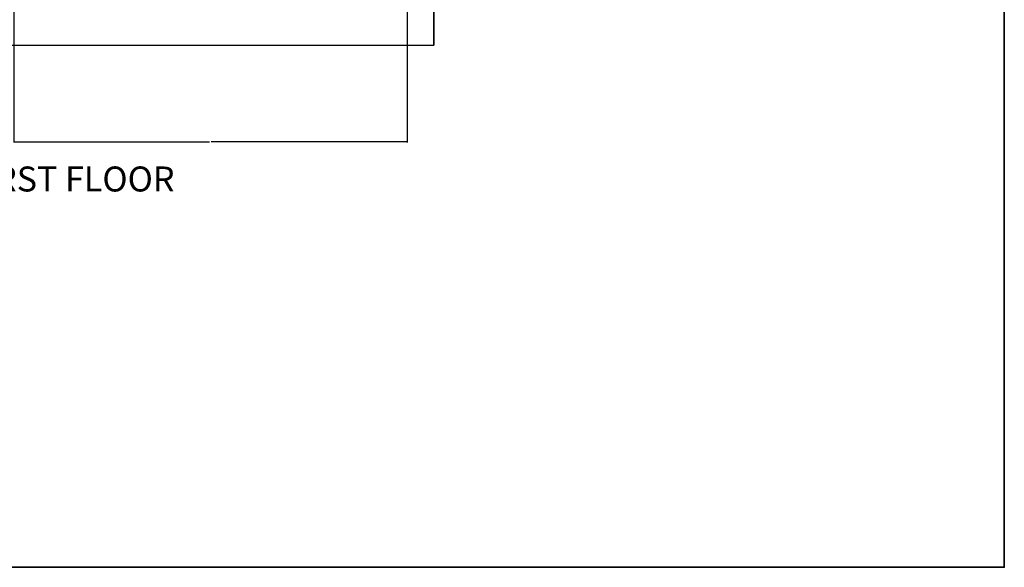
# Model space of a CAD drawing. Units: feet. Extents: x 1654 to 2985, y 1348 to 2230.
# Tile 42 of 53: x 2655 to 2985, y 1348 to 1532. Entities that reach past the tile are written whole.
import ezdxf

# ---------------------------------------------------------------- set-up
doc = ezdxf.new("R2010")
doc.units = ezdxf.units.FT
for name, color, linetype, lineweight in [('A-ANNO-DIMS', 2, 'Continuous', 18), ('A-ANNO-TITL', 7, 'Continuous', 35), ('A-ANNO-TTLB', 7, 'Continuous', 35), ('A-FLOR', 7, 'Continuous', 25), ('A-WALL', 7, 'Continuous', 35)]:
    doc.layers.add(name, color=color, linetype=linetype, lineweight=lineweight)
doc.styles.get("Standard").update_dxf_attribs({"font": 'arial.ttf'})
doc.dimstyles.get("Standard").update_dxf_attribs({"dimtxt": 0.18, "dimasz": 0.18, "dimexe": 0.18, "dimexo": 0.0625, "dimgap": 0.09, "dimtad": 0, "dimtih": 1, "dimtoh": 1, "dimdec": 4, "dimzin": 0, "dimdsep": 46, "dimtxsty": 'Standard', "dimcen": 0.09, "dimadec": 0, "dimazin": 0, "dimtfac": 1, "dimtdec": 4, "dimtofl": 0, "dimtmove": 0, "dimatfit": 3, "dimfxl": 1, "dimtolj": 1, "dimtzin": 0, "dimarcsym": 0})

# ---------------------------------------------------------------- blocks, each defined once
blk = doc.blocks.new('*D82')
at = {"layer": 'A-ANNO-DIMS', "color": 0, "lineweight": -2, "transparency": 16777216}
for p, q in [((2652.71, 2039.19), (2652.71, 1490.62)), ((2784.71, 2039.19), (2784.71, 1490.62)), ((2652.89, 1490.8), (2718.43, 1490.8)), ((2784.53, 1490.8), (2718.99, 1490.8))]:
    blk.add_line(p, q, dxfattribs=at)
at = {"layer": 'A-ANNO-DIMS', "color": 0, "transparency": 16777216}
for points in [[(2652.89, 1490.83), (2652.89, 1490.77), (2652.71, 1490.8)], [(2784.53, 1490.83), (2784.53, 1490.77), (2784.71, 1490.8)]]:
    blk.add_solid(points, dxfattribs=at)
at = {"layer": 'Defpoints', "color": 0, "transparency": 16777216}
for p in [(2652.71, 2039.25), (2784.71, 2039.25), (2784.71, 1490.8)]:
    blk.add_point(p, dxfattribs=at)
at = {"layer": 'A-ANNO-DIMS', "color": 0, "transparency": 16777216, "insert": (2718.71, 1490.8), "char_height": 0.18, "attachment_point": 5}
blk.add_mtext('\\A1;132', dxfattribs=at)

msp = doc.modelspace()

# ---------------------------------------------------------------- linework, layer by layer
at = {"layer": 'A-ANNO-TTLB'}
msp.add_lwpolyline([(1654.1997, 2230.0267), (2985.175, 2230.0267), (2985.175, 1348.1324), (1654.1997, 1348.1324)], close=True, dxfattribs=at)
at = {"layer": 'A-FLOR'}
msp.add_line((2425.7058, 1523.2549), (2793.7058, 1523.2549), dxfattribs=at)
at = {"layer": 'A-WALL'}
msp.add_line((2793.7058, 1886.2549), (2793.7058, 1523.2549), dxfattribs=at)

# ---------------------------------------------------------------- texts
at = {"layer": 'A-ANNO-TITL'}
msp.add_text('FIRST FLOOR', height=8.38114, dxfattribs=at).set_placement((2636.7843, 1474.1641))

# ---------------------------------------------------------------- dimensions: what is measured, and where the dimension line sits
at = {"layer": 'A-ANNO-DIMS'}
dim = msp.add_linear_dim(base=(2784.7058, 1490.8049), p1=(2652.7058, 2039.2549), p2=(2784.7058, 2039.2549), dimstyle='Standard', override={"dimdec": 0, "dimlfac": 1, "dimrnd": 0, "dimzin": 0, "dimdsep": 46, "dimlunit": 2}, dxfattribs=at)
dim.commit()
dim.dimension.update_dxf_attribs({"geometry": '*D82', "text_midpoint": (2718.7058, 1490.8049)})

doc.saveas('drawing.dxf')
